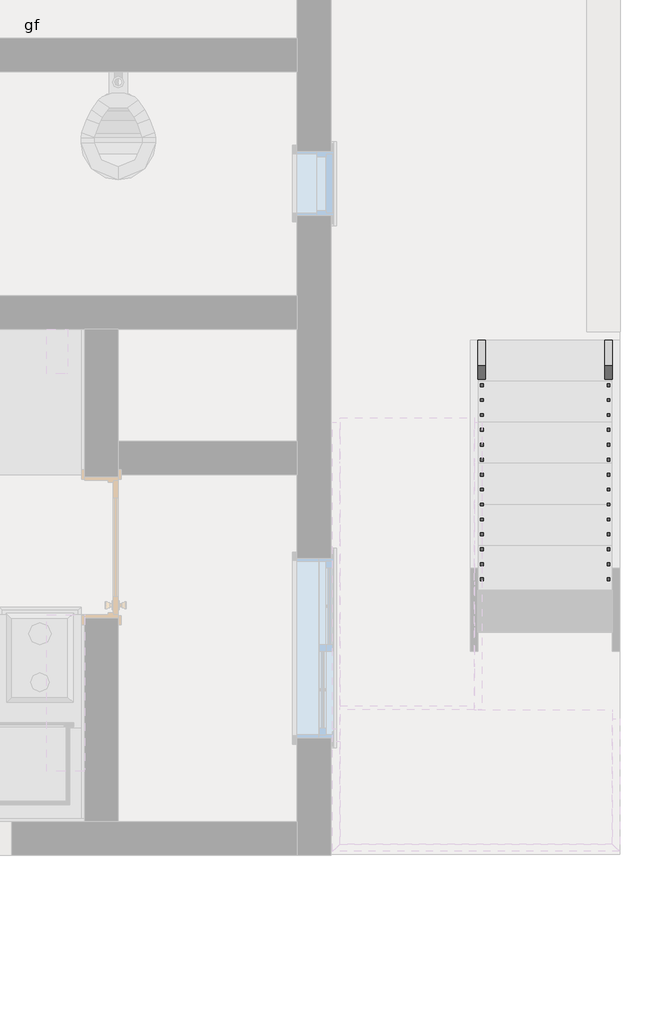
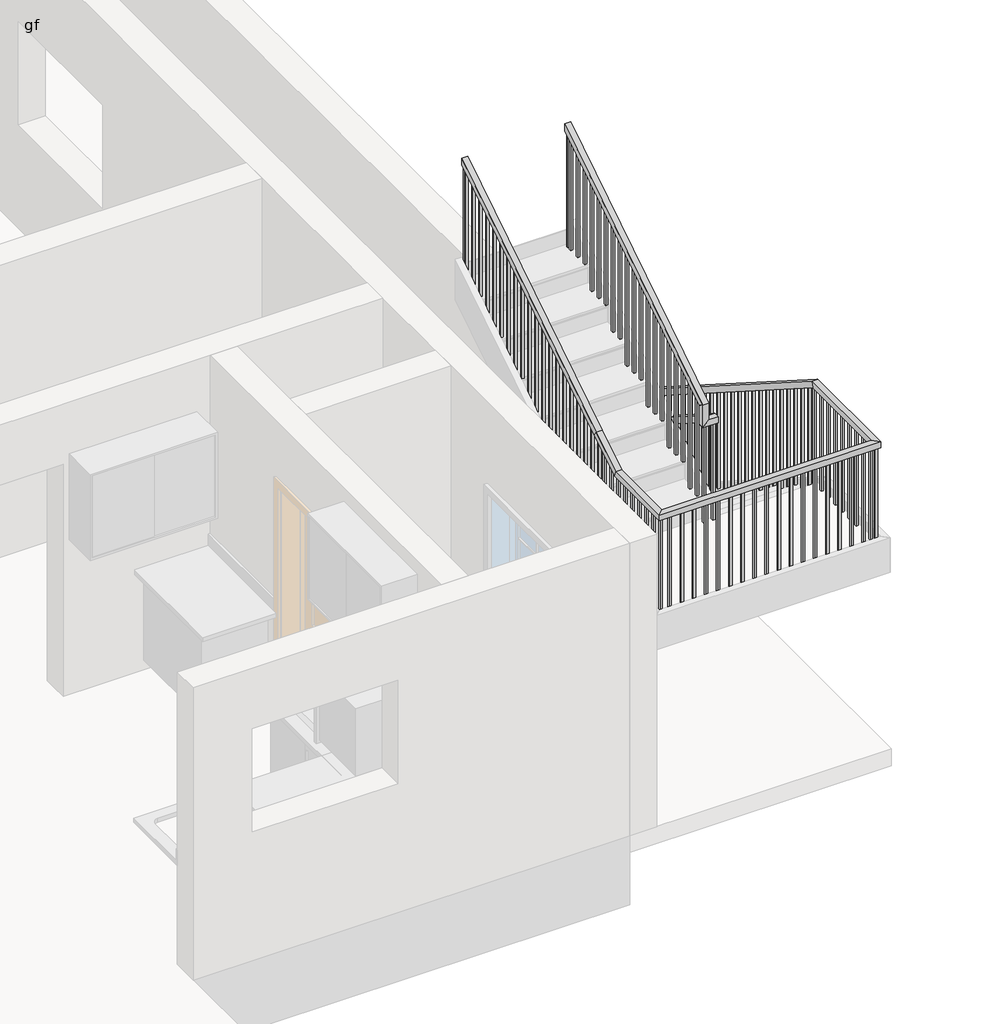
# One storey, part 6 of 8: 2 railings.
"""IFC4 building model written with IfcOpenShell, lengths in millimetres."""

from ifc_helpers import new_model, si_unit, frame, origin, place, context, project, spatial, polyline, outline, extrude, faceted_brep, element, save

model = new_model("IFC4")

# Units and contexts
model_context = context("Model", 3, world=origin())
ifc_project = project(units=[si_unit("LENGTHUNIT", "METRE", prefix="MILLI")], contexts=[model_context])

# Site, building, storey
site = spatial("IfcSite", under=ifc_project)
building = spatial("IfcBuilding", under=site)
storey = spatial("IfcBuildingStorey", under=building, Name="gf", Elevation=609.6)

# Railings
placement = place(None, origin())
element("IfcRailing", 1, ObjectType="Handrail - Rectangular", at=placement, inside=storey, context=model_context, shape_type="SolidModel", body=[
    faceted_brep([(14286.6761273, -1100.1064015, 1701.8), (14286.6761273, -1100.1064015, 1641.586276), (14235.8761273, -1100.1064015, 1641.586276), (14235.8761273, -1100.1064015, 1701.8), (14286.6761273, -3614.7064015, 3302.0), (14235.8761273, -3614.7064015, 3302.0), (14235.8761273, -3614.7064015, 3241.786276), (14286.6761273, -3614.7064015, 3241.786276)], [[[0, 1, 2, 3]], [[4, 5, 6, 7]], [[1, 0, 4, 7]], [[2, 1, 7, 6]], [[3, 2, 6, 5]], [[0, 3, 5, 4]]]),
    faceted_brep([(14286.6761273, -3665.5064015, 3302.0), (14286.6761273, -3665.5064015, 3251.2), (14286.6761273, -3614.7064015, 3251.2), (14286.6761273, -3614.7064015, 3302.0), (14210.4761273, -3665.5064015, 3302.0), (14210.4761273, -3614.7064015, 3302.0), (14159.6761273, -3614.7064015, 3251.2), (14159.6761273, -3665.5064015, 3251.2)], [[[0, 1, 2, 3]], [[4, 5, 6, 7]], [[1, 0, 4, 7]], [[2, 1, 7, 6]], [[3, 2, 6, 5]], [[0, 3, 5, 4]]]),
    faceted_brep([(14210.4761273, -3665.5064015, 3302.0), (14159.6761273, -3665.5064015, 3251.2), (14159.6761273, -3614.7064015, 3251.2), (14210.4761273, -3614.7064015, 3302.0), (14210.4761273, -3665.5064015, 3447.4727273), (14210.4761273, -3614.7064015, 3419.586276), (14159.6761273, -3614.7064015, 3419.586276), (14159.6761273, -3665.5064015, 3447.4727273)], [[[0, 1, 2, 3]], [[4, 5, 6, 7]], [[1, 0, 4, 7]], [[2, 1, 7, 6]], [[3, 2, 6, 5]], [[0, 3, 5, 4]]]),
    faceted_brep([(14159.6761273, -3665.5064015, 3447.4727273), (14159.6761273, -3614.7064015, 3419.586276), (14210.4761273, -3614.7064015, 3419.586276), (14210.4761273, -3665.5064015, 3447.4727273), (14159.6761273, -1658.9064015, 4724.4), (14210.4761273, -1658.9064015, 4724.4), (14210.4761273, -1658.9064015, 4664.186276), (14159.6761273, -1658.9064015, 4664.186276)], [[[0, 1, 2, 3]], [[4, 5, 6, 7]], [[1, 0, 4, 7]], [[2, 1, 7, 6]], [[3, 2, 6, 5]], [[0, 3, 5, 4]]]),
    extrude(outline(polyline([(-1719.2314015, 4625.7976396), (-1700.1814015, 4637.9203669), (-1700.1814015, 3632.2), (-1719.2314015, 3632.2), (-1719.2314015, 4625.7976396)])), frame((14175.5511273, 0.0, 0.0), z_axis=(1.0, 0.0, 0.0), x_axis=(0.0, 1.0, 0.0)), (0.0, 0.0, 1.0), 19.05),
    extrude(outline(polyline([(-1820.8314015, 4561.1430941), (-1801.7814015, 4573.2658214), (-1801.7814015, 3632.2), (-1820.8314015, 3632.2), (-1820.8314015, 4561.1430941)])), frame((14175.5511273, 0.0, 0.0), z_axis=(1.0, 0.0, 0.0), x_axis=(0.0, 1.0, 0.0)), (0.0, 0.0, 1.0), 19.05),
    extrude(outline(polyline([(-1922.4314015, 4496.4885487), (-1903.3814015, 4508.611276), (-1903.3814015, 3632.2), (-1922.4314015, 3632.2), (-1922.4314015, 4496.4885487)])), frame((14175.5511273, 0.0, 0.0), z_axis=(1.0, 0.0, 0.0), x_axis=(0.0, 1.0, 0.0)), (0.0, 0.0, 1.0), 19.05),
    extrude(outline(polyline([(-2024.0314015, 4431.8340032), (-2004.9814015, 4443.9567305), (-2004.9814015, 3454.4), (-2024.0314015, 3454.4), (-2024.0314015, 4431.8340032)])), frame((14175.5511273, 0.0, 0.0), z_axis=(1.0, 0.0, 0.0), x_axis=(0.0, 1.0, 0.0)), (0.0, 0.0, 1.0), 19.05),
    extrude(outline(polyline([(-2125.6314015, 4367.1794578), (-2106.5814015, 4379.3021851), (-2106.5814015, 3454.4), (-2125.6314015, 3454.4), (-2125.6314015, 4367.1794578)])), frame((14175.5511273, 0.0, 0.0), z_axis=(1.0, 0.0, 0.0), x_axis=(0.0, 1.0, 0.0)), (0.0, 0.0, 1.0), 19.05),
    extrude(outline(polyline([(-2227.2314015, 4302.5249123), (-2208.1814015, 4314.6476396), (-2208.1814015, 3454.4), (-2227.2314015, 3454.4), (-2227.2314015, 4302.5249123)])), frame((14175.5511273, 0.0, 0.0), z_axis=(1.0, 0.0, 0.0), x_axis=(0.0, 1.0, 0.0)), (0.0, 0.0, 1.0), 19.05),
    extrude(outline(polyline([(-2328.8314015, 4237.8703669), (-2309.7814015, 4249.9930941), (-2309.7814015, 3276.6), (-2328.8314015, 3276.6), (-2328.8314015, 4237.8703669)])), frame((14175.5511273, 0.0, 0.0), z_axis=(1.0, 0.0, 0.0), x_axis=(0.0, 1.0, 0.0)), (0.0, 0.0, 1.0), 19.05),
    extrude(outline(polyline([(-2430.4314015, 4173.2158214), (-2411.3814015, 4185.3385487), (-2411.3814015, 3276.6), (-2430.4314015, 3276.6), (-2430.4314015, 4173.2158214)])), frame((14175.5511273, 0.0, 0.0), z_axis=(1.0, 0.0, 0.0), x_axis=(0.0, 1.0, 0.0)), (0.0, 0.0, 1.0), 19.05),
    extrude(outline(polyline([(-2532.0314015, 4108.561276), (-2512.9814015, 4120.6840032), (-2512.9814015, 3098.8), (-2532.0314015, 3098.8), (-2532.0314015, 4108.561276)])), frame((14175.5511273, 0.0, 0.0), z_axis=(1.0, 0.0, 0.0), x_axis=(0.0, 1.0, 0.0)), (0.0, 0.0, 1.0), 19.05),
    extrude(outline(polyline([(-2633.6314015, 4043.9067305), (-2614.5814015, 4056.0294578), (-2614.5814015, 3098.8), (-2633.6314015, 3098.8), (-2633.6314015, 4043.9067305)])), frame((14175.5511273, 0.0, 0.0), z_axis=(1.0, 0.0, 0.0), x_axis=(0.0, 1.0, 0.0)), (0.0, 0.0, 1.0), 19.05),
    extrude(outline(polyline([(-2735.2314015, 3979.2521851), (-2716.1814015, 3991.3749123), (-2716.1814015, 3098.8), (-2735.2314015, 3098.8), (-2735.2314015, 3979.2521851)])), frame((14175.5511273, 0.0, 0.0), z_axis=(1.0, 0.0, 0.0), x_axis=(0.0, 1.0, 0.0)), (0.0, 0.0, 1.0), 19.05),
    extrude(outline(polyline([(-2836.8314015, 3914.5976396), (-2817.7814015, 3926.7203669), (-2817.7814015, 2921.0), (-2836.8314015, 2921.0), (-2836.8314015, 3914.5976396)])), frame((14175.5511273, 0.0, 0.0), z_axis=(1.0, 0.0, 0.0), x_axis=(0.0, 1.0, 0.0)), (0.0, 0.0, 1.0), 19.05),
    extrude(outline(polyline([(-2938.4314015, 3849.9430941), (-2919.3814015, 3862.0658214), (-2919.3814015, 2921.0), (-2938.4314015, 2921.0), (-2938.4314015, 3849.9430941)])), frame((14175.5511273, 0.0, 0.0), z_axis=(1.0, 0.0, 0.0), x_axis=(0.0, 1.0, 0.0)), (0.0, 0.0, 1.0), 19.05),
    extrude(outline(polyline([(-3040.0314015, 3785.2885487), (-3020.9814015, 3797.411276), (-3020.9814015, 2921.0), (-3040.0314015, 2921.0), (-3040.0314015, 3785.2885487)])), frame((14175.5511273, 0.0, 0.0), z_axis=(1.0, 0.0, 0.0), x_axis=(0.0, 1.0, 0.0)), (0.0, 0.0, 1.0), 19.05),
    extrude(outline(polyline([(-3141.6314015, 3720.6340032), (-3122.5814015, 3732.7567305), (-3122.5814015, 2743.2), (-3141.6314015, 2743.2), (-3141.6314015, 3720.6340032)])), frame((14175.5511273, 0.0, 0.0), z_axis=(1.0, 0.0, 0.0), x_axis=(0.0, 1.0, 0.0)), (0.0, 0.0, 1.0), 19.05),
    extrude(outline(polyline([(-3243.2314015, 3655.9794578), (-3224.1814015, 3668.1021851), (-3224.1814015, 2743.2), (-3243.2314015, 2743.2), (-3243.2314015, 3655.9794578)])), frame((14175.5511273, 0.0, 0.0), z_axis=(1.0, 0.0, 0.0), x_axis=(0.0, 1.0, 0.0)), (0.0, 0.0, 1.0), 19.05),
    extrude(outline(polyline([(-3344.8314015, 3591.3249123), (-3325.7814015, 3603.4476396), (-3325.7814015, 2743.2), (-3344.8314015, 2743.2), (-3344.8314015, 3591.3249123)])), frame((14175.5511273, 0.0, 0.0), z_axis=(1.0, 0.0, 0.0), x_axis=(0.0, 1.0, 0.0)), (0.0, 0.0, 1.0), 19.05),
    extrude(outline(polyline([(-3446.4314015, 3526.6703669), (-3427.3814015, 3538.7930941), (-3427.3814015, 2565.4), (-3446.4314015, 2565.4), (-3446.4314015, 3526.6703669)])), frame((14175.5511273, 0.0, 0.0), z_axis=(1.0, 0.0, 0.0), x_axis=(0.0, 1.0, 0.0)), (0.0, 0.0, 1.0), 19.05),
    extrude(outline(polyline([(-3548.0314015, 3462.0158214), (-3528.9814015, 3474.1385487), (-3528.9814015, 2565.4), (-3548.0314015, 2565.4), (-3548.0314015, 3462.0158214)])), frame((14175.5511273, 0.0, 0.0), z_axis=(1.0, 0.0, 0.0), x_axis=(0.0, 1.0, 0.0)), (0.0, 0.0, 1.0), 19.05),
    extrude(outline(polyline([(-3548.0314015, 3199.3567305), (-3528.9814015, 3187.2340032), (-3528.9814015, 2209.8), (-3548.0314015, 2209.8), (-3548.0314015, 3199.3567305)])), frame((14251.7511273, 0.0, 0.0), z_axis=(1.0, 0.0, 0.0), x_axis=(0.0, 1.0, 0.0)), (0.0, 0.0, 1.0), 19.05),
    extrude(outline(polyline([(-3446.4314015, 3134.7021851), (-3427.3814015, 3122.5794578), (-3427.3814015, 2209.8), (-3446.4314015, 2209.8), (-3446.4314015, 3134.7021851)])), frame((14251.7511273, 0.0, 0.0), z_axis=(1.0, 0.0, 0.0), x_axis=(0.0, 1.0, 0.0)), (0.0, 0.0, 1.0), 19.05),
    extrude(outline(polyline([(-3344.8314015, 3070.0476396), (-3325.7814015, 3057.9249123), (-3325.7814015, 2209.8), (-3344.8314015, 2209.8), (-3344.8314015, 3070.0476396)])), frame((14251.7511273, 0.0, 0.0), z_axis=(1.0, 0.0, 0.0), x_axis=(0.0, 1.0, 0.0)), (0.0, 0.0, 1.0), 19.05),
    extrude(outline(polyline([(-3243.2314015, 3005.3930941), (-3224.1814015, 2993.2703669), (-3224.1814015, 2032.0), (-3243.2314015, 2032.0), (-3243.2314015, 3005.3930941)])), frame((14251.7511273, 0.0, 0.0), z_axis=(1.0, 0.0, 0.0), x_axis=(0.0, 1.0, 0.0)), (0.0, 0.0, 1.0), 19.05),
    extrude(outline(polyline([(-3141.6314015, 2940.7385487), (-3122.5814015, 2928.6158214), (-3122.5814015, 2032.0), (-3141.6314015, 2032.0), (-3141.6314015, 2940.7385487)])), frame((14251.7511273, 0.0, 0.0), z_axis=(1.0, 0.0, 0.0), x_axis=(0.0, 1.0, 0.0)), (0.0, 0.0, 1.0), 19.05),
    extrude(outline(polyline([(-3040.0314015, 2876.0840032), (-3020.9814015, 2863.961276), (-3020.9814015, 1854.2), (-3040.0314015, 1854.2), (-3040.0314015, 2876.0840032)])), frame((14251.7511273, 0.0, 0.0), z_axis=(1.0, 0.0, 0.0), x_axis=(0.0, 1.0, 0.0)), (0.0, 0.0, 1.0), 19.05),
    extrude(outline(polyline([(-2938.4314015, 2811.4294578), (-2919.3814015, 2799.3067305), (-2919.3814015, 1854.2), (-2938.4314015, 1854.2), (-2938.4314015, 2811.4294578)])), frame((14251.7511273, 0.0, 0.0), z_axis=(1.0, 0.0, 0.0), x_axis=(0.0, 1.0, 0.0)), (0.0, 0.0, 1.0), 19.05),
    extrude(outline(polyline([(-2836.8314015, 2746.7749123), (-2817.7814015, 2734.6521851), (-2817.7814015, 1854.2), (-2836.8314015, 1854.2), (-2836.8314015, 2746.7749123)])), frame((14251.7511273, 0.0, 0.0), z_axis=(1.0, 0.0, 0.0), x_axis=(0.0, 1.0, 0.0)), (0.0, 0.0, 1.0), 19.05),
    extrude(outline(polyline([(-2735.2314015, 2682.1203669), (-2716.1814015, 2669.9976396), (-2716.1814015, 1676.4), (-2735.2314015, 1676.4), (-2735.2314015, 2682.1203669)])), frame((14251.7511273, 0.0, 0.0), z_axis=(1.0, 0.0, 0.0), x_axis=(0.0, 1.0, 0.0)), (0.0, 0.0, 1.0), 19.05),
    extrude(outline(polyline([(-2633.6314015, 2617.4658214), (-2614.5814015, 2605.3430941), (-2614.5814015, 1676.4), (-2633.6314015, 1676.4), (-2633.6314015, 2617.4658214)])), frame((14251.7511273, 0.0, 0.0), z_axis=(1.0, 0.0, 0.0), x_axis=(0.0, 1.0, 0.0)), (0.0, 0.0, 1.0), 19.05),
    extrude(outline(polyline([(-2532.0314015, 2552.811276), (-2512.9814015, 2540.6885487), (-2512.9814015, 1676.4), (-2532.0314015, 1676.4), (-2532.0314015, 2552.811276)])), frame((14251.7511273, 0.0, 0.0), z_axis=(1.0, 0.0, 0.0), x_axis=(0.0, 1.0, 0.0)), (0.0, 0.0, 1.0), 19.05),
    extrude(outline(polyline([(-2430.4314015, 2488.1567305), (-2411.3814015, 2476.0340032), (-2411.3814015, 1498.6), (-2430.4314015, 1498.6), (-2430.4314015, 2488.1567305)])), frame((14251.7511273, 0.0, 0.0), z_axis=(1.0, 0.0, 0.0), x_axis=(0.0, 1.0, 0.0)), (0.0, 0.0, 1.0), 19.05),
    extrude(outline(polyline([(-2328.8314015, 2423.5021851), (-2309.7814015, 2411.3794578), (-2309.7814015, 1498.6), (-2328.8314015, 1498.6), (-2328.8314015, 2423.5021851)])), frame((14251.7511273, 0.0, 0.0), z_axis=(1.0, 0.0, 0.0), x_axis=(0.0, 1.0, 0.0)), (0.0, 0.0, 1.0), 19.05),
    extrude(outline(polyline([(-2227.2314015, 2358.8476396), (-2208.1814015, 2346.7249123), (-2208.1814015, 1498.6), (-2227.2314015, 1498.6), (-2227.2314015, 2358.8476396)])), frame((14251.7511273, 0.0, 0.0), z_axis=(1.0, 0.0, 0.0), x_axis=(0.0, 1.0, 0.0)), (0.0, 0.0, 1.0), 19.05),
    extrude(outline(polyline([(-2125.6314015, 2294.1930941), (-2106.5814015, 2282.0703669), (-2106.5814015, 1320.8), (-2125.6314015, 1320.8), (-2125.6314015, 2294.1930941)])), frame((14251.7511273, 0.0, 0.0), z_axis=(1.0, 0.0, 0.0), x_axis=(0.0, 1.0, 0.0)), (0.0, 0.0, 1.0), 19.05),
    extrude(outline(polyline([(-2024.0314015, 2229.5385487), (-2004.9814015, 2217.4158214), (-2004.9814015, 1320.8), (-2024.0314015, 1320.8), (-2024.0314015, 2229.5385487)])), frame((14251.7511273, 0.0, 0.0), z_axis=(1.0, 0.0, 0.0), x_axis=(0.0, 1.0, 0.0)), (0.0, 0.0, 1.0), 19.05),
    extrude(outline(polyline([(-1922.4314015, 2164.8840032), (-1903.3814015, 2152.761276), (-1903.3814015, 1143.0), (-1922.4314015, 1143.0), (-1922.4314015, 2164.8840032)])), frame((14251.7511273, 0.0, 0.0), z_axis=(1.0, 0.0, 0.0), x_axis=(0.0, 1.0, 0.0)), (0.0, 0.0, 1.0), 19.05),
    extrude(outline(polyline([(-1820.8314015, 2100.2294578), (-1801.7814015, 2088.1067305), (-1801.7814015, 1143.0), (-1820.8314015, 1143.0), (-1820.8314015, 2100.2294578)])), frame((14251.7511273, 0.0, 0.0), z_axis=(1.0, 0.0, 0.0), x_axis=(0.0, 1.0, 0.0)), (0.0, 0.0, 1.0), 19.05),
    extrude(outline(polyline([(-1719.2314015, 2035.5749123), (-1700.1814015, 2023.4521851), (-1700.1814015, 1143.0), (-1719.2314015, 1143.0), (-1719.2314015, 2035.5749123)])), frame((14251.7511273, 0.0, 0.0), z_axis=(1.0, 0.0, 0.0), x_axis=(0.0, 1.0, 0.0)), (0.0, 0.0, 1.0), 19.05),
    extrude(outline(polyline([(-1617.6314015, 1970.9203669), (-1598.5814015, 1958.7976396), (-1598.5814015, 965.2), (-1617.6314015, 965.2), (-1617.6314015, 1970.9203669)])), frame((14251.7511273, 0.0, 0.0), z_axis=(1.0, 0.0, 0.0), x_axis=(0.0, 1.0, 0.0)), (0.0, 0.0, 1.0), 19.05),
    extrude(outline(polyline([(-1516.0314015, 1906.2658214), (-1496.9814015, 1894.1430941), (-1496.9814015, 965.2), (-1516.0314015, 965.2), (-1516.0314015, 1906.2658214)])), frame((14251.7511273, 0.0, 0.0), z_axis=(1.0, 0.0, 0.0), x_axis=(0.0, 1.0, 0.0)), (0.0, 0.0, 1.0), 19.05),
    extrude(outline(polyline([(-1414.4314015, 1841.611276), (-1395.3814015, 1829.4885487), (-1395.3814015, 965.2), (-1414.4314015, 965.2), (-1414.4314015, 1841.611276)])), frame((14251.7511273, 0.0, 0.0), z_axis=(1.0, 0.0, 0.0), x_axis=(0.0, 1.0, 0.0)), (0.0, 0.0, 1.0), 19.05),
    extrude(outline(polyline([(-1312.8314015, 1776.9567305), (-1293.7814015, 1764.8340032), (-1293.7814015, 787.4), (-1312.8314015, 787.4), (-1312.8314015, 1776.9567305)])), frame((14251.7511273, 0.0, 0.0), z_axis=(1.0, 0.0, 0.0), x_axis=(0.0, 1.0, 0.0)), (0.0, 0.0, 1.0), 19.05),
    extrude(outline(polyline([(-1211.2314015, 1712.3021851), (-1192.1814015, 1700.1794578), (-1192.1814015, 787.4), (-1211.2314015, 787.4), (-1211.2314015, 1712.3021851)])), frame((14251.7511273, 0.0, 0.0), z_axis=(1.0, 0.0, 0.0), x_axis=(0.0, 1.0, 0.0)), (0.0, 0.0, 1.0), 19.05),
    extrude(outline(polyline([(14194.6011273, -3630.5814015), (14194.6011273, -3649.6314015), (14175.5511273, -3649.6314015), (14175.5511273, -3630.5814015), (14194.6011273, -3630.5814015)])), frame((0.0, 0.0, 2387.6), z_axis=(0.0, 0.0, 1.0), x_axis=(1.0, 0.0, 0.0)), (0.0, 0.0, 1.0), 863.6),
    extrude(outline(polyline([(-3649.6314015, 3264.011276), (-3630.5814015, 3251.8885487), (-3630.5814015, 2387.6), (-3649.6314015, 2387.6), (-3649.6314015, 3264.011276)])), frame((14251.7511273, 0.0, 0.0), z_axis=(1.0, 0.0, 0.0), x_axis=(0.0, 1.0, 0.0)), (0.0, 0.0, 1.0), 19.05),
    extrude(outline(polyline([(-1677.9564015, 4652.0635487), (-1658.9064015, 4664.186276), (-1658.9064015, 3632.2), (-1677.9564015, 3632.2), (-1677.9564015, 4652.0635487)])), frame((14175.5511273, 0.0, 0.0), z_axis=(1.0, 0.0, 0.0), x_axis=(0.0, 1.0, 0.0)), (0.0, 0.0, 1.0), 19.05),
    extrude(outline(polyline([(-1119.1564015, 1653.7090032), (-1100.1064015, 1641.586276), (-1100.1064015, 787.4), (-1119.1564015, 787.4), (-1119.1564015, 1653.7090032)])), frame((14251.7511273, 0.0, 0.0), z_axis=(1.0, 0.0, 0.0), x_axis=(0.0, 1.0, 0.0)), (0.0, 0.0, 1.0), 19.05),
])
element("IfcRailing", 2, ObjectType="Handrail - Rectangular", at=placement, inside=storey, context=model_context, shape_type="SolidModel", body=[
    faceted_brep([(15150.2761273, -1100.1064015, 1701.8), (15150.2761273, -1100.1064015, 1641.586276), (15099.4761273, -1100.1064015, 1641.586276), (15099.4761273, -1100.1064015, 1701.8), (15150.2761273, -3614.7064015, 3302.0), (15150.2761273, -3629.4993964, 3251.2), (15099.4761273, -3629.4993964, 3251.2), (15099.4761273, -3614.7064015, 3302.0), (15150.2761273, -4529.1064015, 3302.0), (15150.2761273, -4529.1064015, 3251.2), (15099.4761273, -4478.3064015, 3251.2), (15099.4761273, -4478.3064015, 3302.0), (13296.0761273, -4529.1064015, 3302.0), (13296.0761273, -4529.1064015, 3251.2), (13346.8761273, -4478.3064015, 3251.2), (13346.8761273, -4478.3064015, 3302.0), (13296.0761273, -3894.1064015, 3302.0), (13296.0761273, -3879.3134066, 3251.2), (13346.8761273, -3879.3134066, 3251.2), (13346.8761273, -3894.1064015, 3302.0), (13296.0761273, -3614.7064015, 3479.8), (13296.0761273, -3587.4331265, 3436.9419964), (13346.8761273, -3587.4331265, 3436.9419964), (13346.8761273, -3614.7064015, 3479.8), (13296.0761273, -1658.9064015, 4724.4), (13346.8761273, -1658.9064015, 4724.4), (13346.8761273, -1658.9064015, 4664.186276), (13296.0761273, -1658.9064015, 4664.186276)], [[[0, 1, 2, 3]], [[1, 0, 4, 5]], [[2, 1, 5, 6]], [[3, 2, 6, 7]], [[0, 3, 7, 4]], [[5, 4, 8, 9]], [[6, 5, 9, 10]], [[7, 6, 10, 11]], [[4, 7, 11, 8]], [[9, 8, 12, 13]], [[10, 9, 13, 14]], [[11, 10, 14, 15]], [[8, 11, 15, 12]], [[13, 12, 16, 17]], [[14, 13, 17, 18]], [[15, 14, 18, 19]], [[12, 15, 19, 16]], [[17, 16, 20, 21]], [[18, 17, 21, 22]], [[19, 18, 22, 23]], [[16, 19, 23, 20]], [[24, 25, 26, 27]], [[21, 20, 24, 27]], [[22, 21, 27, 26]], [[23, 22, 26, 25]], [[20, 23, 25, 24]]]),
    extrude(outline(polyline([(-1674.7814015, 4654.0840032), (-1674.7814015, 3632.2), (-1693.8314015, 3632.2), (-1693.8314015, 4641.961276), (-1674.7814015, 4654.0840032)])), frame((13311.9511273, 0.0, 0.0), z_axis=(1.0, 0.0, 0.0), x_axis=(0.0, 1.0, 0.0)), (0.0, 0.0, 1.0), 19.05),
    extrude(outline(polyline([(-1776.3814015, 4589.4294578), (-1776.3814015, 3632.2), (-1795.4314015, 3632.2), (-1795.4314015, 4577.3067305), (-1776.3814015, 4589.4294578)])), frame((13311.9511273, 0.0, 0.0), z_axis=(1.0, 0.0, 0.0), x_axis=(0.0, 1.0, 0.0)), (0.0, 0.0, 1.0), 19.05),
    extrude(outline(polyline([(-1877.9814015, 4524.7749123), (-1877.9814015, 3632.2), (-1897.0314015, 3632.2), (-1897.0314015, 4512.6521851), (-1877.9814015, 4524.7749123)])), frame((13311.9511273, 0.0, 0.0), z_axis=(1.0, 0.0, 0.0), x_axis=(0.0, 1.0, 0.0)), (0.0, 0.0, 1.0), 19.05),
    extrude(outline(polyline([(-1979.5814015, 4460.1203669), (-1979.5814015, 3454.4), (-1998.6314015, 3454.4), (-1998.6314015, 4447.9976396), (-1979.5814015, 4460.1203669)])), frame((13311.9511273, 0.0, 0.0), z_axis=(1.0, 0.0, 0.0), x_axis=(0.0, 1.0, 0.0)), (0.0, 0.0, 1.0), 19.05),
    extrude(outline(polyline([(-2081.1814015, 4395.4658214), (-2081.1814015, 3454.4), (-2100.2314015, 3454.4), (-2100.2314015, 4383.3430941), (-2081.1814015, 4395.4658214)])), frame((13311.9511273, 0.0, 0.0), z_axis=(1.0, 0.0, 0.0), x_axis=(0.0, 1.0, 0.0)), (0.0, 0.0, 1.0), 19.05),
    extrude(outline(polyline([(-2182.7814015, 4330.811276), (-2182.7814015, 3454.4), (-2201.8314015, 3454.4), (-2201.8314015, 4318.6885487), (-2182.7814015, 4330.811276)])), frame((13311.9511273, 0.0, 0.0), z_axis=(1.0, 0.0, 0.0), x_axis=(0.0, 1.0, 0.0)), (0.0, 0.0, 1.0), 19.05),
    extrude(outline(polyline([(-2284.3814015, 4266.1567305), (-2284.3814015, 3276.6), (-2303.4314015, 3276.6), (-2303.4314015, 4254.0340032), (-2284.3814015, 4266.1567305)])), frame((13311.9511273, 0.0, 0.0), z_axis=(1.0, 0.0, 0.0), x_axis=(0.0, 1.0, 0.0)), (0.0, 0.0, 1.0), 19.05),
    extrude(outline(polyline([(-2385.9814015, 4201.5021851), (-2385.9814015, 3276.6), (-2405.0314015, 3276.6), (-2405.0314015, 4189.3794578), (-2385.9814015, 4201.5021851)])), frame((13311.9511273, 0.0, 0.0), z_axis=(1.0, 0.0, 0.0), x_axis=(0.0, 1.0, 0.0)), (0.0, 0.0, 1.0), 19.05),
    extrude(outline(polyline([(-2487.5814015, 4136.8476396), (-2487.5814015, 3276.6), (-2506.6314015, 3276.6), (-2506.6314015, 4124.7249123), (-2487.5814015, 4136.8476396)])), frame((13311.9511273, 0.0, 0.0), z_axis=(1.0, 0.0, 0.0), x_axis=(0.0, 1.0, 0.0)), (0.0, 0.0, 1.0), 19.05),
    extrude(outline(polyline([(-2589.1814015, 4072.1930941), (-2589.1814015, 3098.8), (-2608.2314015, 3098.8), (-2608.2314015, 4060.0703669), (-2589.1814015, 4072.1930941)])), frame((13311.9511273, 0.0, 0.0), z_axis=(1.0, 0.0, 0.0), x_axis=(0.0, 1.0, 0.0)), (0.0, 0.0, 1.0), 19.05),
    extrude(outline(polyline([(-2690.7814015, 4007.5385487), (-2690.7814015, 3098.8), (-2709.8314015, 3098.8), (-2709.8314015, 3995.4158214), (-2690.7814015, 4007.5385487)])), frame((13311.9511273, 0.0, 0.0), z_axis=(1.0, 0.0, 0.0), x_axis=(0.0, 1.0, 0.0)), (0.0, 0.0, 1.0), 19.05),
    extrude(outline(polyline([(-2792.3814015, 3942.8840032), (-2792.3814015, 2921.0), (-2811.4314015, 2921.0), (-2811.4314015, 3930.761276), (-2792.3814015, 3942.8840032)])), frame((13311.9511273, 0.0, 0.0), z_axis=(1.0, 0.0, 0.0), x_axis=(0.0, 1.0, 0.0)), (0.0, 0.0, 1.0), 19.05),
    extrude(outline(polyline([(-2893.9814015, 3878.2294578), (-2893.9814015, 2921.0), (-2913.0314015, 2921.0), (-2913.0314015, 3866.1067305), (-2893.9814015, 3878.2294578)])), frame((13311.9511273, 0.0, 0.0), z_axis=(1.0, 0.0, 0.0), x_axis=(0.0, 1.0, 0.0)), (0.0, 0.0, 1.0), 19.05),
    extrude(outline(polyline([(-2995.5814015, 3813.5749123), (-2995.5814015, 2921.0), (-3014.6314015, 2921.0), (-3014.6314015, 3801.4521851), (-2995.5814015, 3813.5749123)])), frame((13311.9511273, 0.0, 0.0), z_axis=(1.0, 0.0, 0.0), x_axis=(0.0, 1.0, 0.0)), (0.0, 0.0, 1.0), 19.05),
    extrude(outline(polyline([(-3097.1814015, 3748.9203669), (-3097.1814015, 2743.2), (-3116.2314015, 2743.2), (-3116.2314015, 3736.7976396), (-3097.1814015, 3748.9203669)])), frame((13311.9511273, 0.0, 0.0), z_axis=(1.0, 0.0, 0.0), x_axis=(0.0, 1.0, 0.0)), (0.0, 0.0, 1.0), 19.05),
    extrude(outline(polyline([(-3198.7814015, 3684.2658214), (-3198.7814015, 2743.2), (-3217.8314015, 2743.2), (-3217.8314015, 3672.1430941), (-3198.7814015, 3684.2658214)])), frame((13311.9511273, 0.0, 0.0), z_axis=(1.0, 0.0, 0.0), x_axis=(0.0, 1.0, 0.0)), (0.0, 0.0, 1.0), 19.05),
    extrude(outline(polyline([(-3300.3814015, 3619.611276), (-3300.3814015, 2743.2), (-3319.4314015, 2743.2), (-3319.4314015, 3607.4885487), (-3300.3814015, 3619.611276)])), frame((13311.9511273, 0.0, 0.0), z_axis=(1.0, 0.0, 0.0), x_axis=(0.0, 1.0, 0.0)), (0.0, 0.0, 1.0), 19.05),
    extrude(outline(polyline([(-3401.9814015, 3554.9567305), (-3401.9814015, 2565.4), (-3421.0314015, 2565.4), (-3421.0314015, 3542.8340032), (-3401.9814015, 3554.9567305)])), frame((13311.9511273, 0.0, 0.0), z_axis=(1.0, 0.0, 0.0), x_axis=(0.0, 1.0, 0.0)), (0.0, 0.0, 1.0), 19.05),
    extrude(outline(polyline([(-3503.5814015, 3490.3021851), (-3503.5814015, 2565.4), (-3522.6314015, 2565.4), (-3522.6314015, 3478.1794578), (-3503.5814015, 3490.3021851)])), frame((13311.9511273, 0.0, 0.0), z_axis=(1.0, 0.0, 0.0), x_axis=(0.0, 1.0, 0.0)), (0.0, 0.0, 1.0), 19.05),
    extrude(outline(polyline([(-3681.3814015, 3377.1567305), (-3681.3814015, 2387.6), (-3700.4314015, 2387.6), (-3700.4314015, 3365.0340032), (-3681.3814015, 3377.1567305)])), frame((13311.9511273, 0.0, 0.0), z_axis=(1.0, 0.0, 0.0), x_axis=(0.0, 1.0, 0.0)), (0.0, 0.0, 1.0), 19.05),
    extrude(outline(polyline([(-3782.9814015, 3312.5021851), (-3782.9814015, 2387.6), (-3802.0314015, 2387.6), (-3802.0314015, 3300.3794578), (-3782.9814015, 3312.5021851)])), frame((13311.9511273, 0.0, 0.0), z_axis=(1.0, 0.0, 0.0), x_axis=(0.0, 1.0, 0.0)), (0.0, 0.0, 1.0), 19.05),
    extrude(outline(polyline([(13311.9511273, -3903.6314015), (13311.9511273, -3884.5814015), (13331.0011273, -3884.5814015), (13331.0011273, -3903.6314015), (13311.9511273, -3903.6314015)])), frame((0.0, 0.0, 2387.6), z_axis=(0.0, 0.0, 1.0), x_axis=(1.0, 0.0, 0.0)), (0.0, 0.0, 1.0), 863.6),
    extrude(outline(polyline([(13311.9511273, -4005.2314015), (13311.9511273, -3986.1814015), (13331.0011273, -3986.1814015), (13331.0011273, -4005.2314015), (13311.9511273, -4005.2314015)])), frame((0.0, 0.0, 2387.6), z_axis=(0.0, 0.0, 1.0), x_axis=(1.0, 0.0, 0.0)), (0.0, 0.0, 1.0), 863.6),
    extrude(outline(polyline([(13311.9511273, -4106.8314015), (13311.9511273, -4087.7814015), (13331.0011273, -4087.7814015), (13331.0011273, -4106.8314015), (13311.9511273, -4106.8314015)])), frame((0.0, 0.0, 2387.6), z_axis=(0.0, 0.0, 1.0), x_axis=(1.0, 0.0, 0.0)), (0.0, 0.0, 1.0), 863.6),
    extrude(outline(polyline([(13311.9511273, -4208.4314015), (13311.9511273, -4189.3814015), (13331.0011273, -4189.3814015), (13331.0011273, -4208.4314015), (13311.9511273, -4208.4314015)])), frame((0.0, 0.0, 2387.6), z_axis=(0.0, 0.0, 1.0), x_axis=(1.0, 0.0, 0.0)), (0.0, 0.0, 1.0), 863.6),
    extrude(outline(polyline([(13311.9511273, -4310.0314015), (13311.9511273, -4290.9814015), (13331.0011273, -4290.9814015), (13331.0011273, -4310.0314015), (13311.9511273, -4310.0314015)])), frame((0.0, 0.0, 2387.6), z_axis=(0.0, 0.0, 1.0), x_axis=(1.0, 0.0, 0.0)), (0.0, 0.0, 1.0), 863.6),
    extrude(outline(polyline([(13311.9511273, -4411.6314015), (13311.9511273, -4392.5814015), (13331.0011273, -4392.5814015), (13331.0011273, -4411.6314015), (13311.9511273, -4411.6314015)])), frame((0.0, 0.0, 2387.6), z_axis=(0.0, 0.0, 1.0), x_axis=(1.0, 0.0, 0.0)), (0.0, 0.0, 1.0), 863.6),
    extrude(outline(polyline([(13407.2011273, -4513.2314015), (13388.1511273, -4513.2314015), (13388.1511273, -4494.1814015), (13407.2011273, -4494.1814015), (13407.2011273, -4513.2314015)])), frame((0.0, 0.0, 2387.6), z_axis=(0.0, 0.0, 1.0), x_axis=(1.0, 0.0, 0.0)), (0.0, 0.0, 1.0), 863.6),
    extrude(outline(polyline([(13508.8011273, -4513.2314015), (13489.7511273, -4513.2314015), (13489.7511273, -4494.1814015), (13508.8011273, -4494.1814015), (13508.8011273, -4513.2314015)])), frame((0.0, 0.0, 2387.6), z_axis=(0.0, 0.0, 1.0), x_axis=(1.0, 0.0, 0.0)), (0.0, 0.0, 1.0), 863.6),
    extrude(outline(polyline([(13610.4011273, -4513.2314015), (13591.3511273, -4513.2314015), (13591.3511273, -4494.1814015), (13610.4011273, -4494.1814015), (13610.4011273, -4513.2314015)])), frame((0.0, 0.0, 2387.6), z_axis=(0.0, 0.0, 1.0), x_axis=(1.0, 0.0, 0.0)), (0.0, 0.0, 1.0), 863.6),
    extrude(outline(polyline([(13712.0011273, -4513.2314015), (13692.9511273, -4513.2314015), (13692.9511273, -4494.1814015), (13712.0011273, -4494.1814015), (13712.0011273, -4513.2314015)])), frame((0.0, 0.0, 2387.6), z_axis=(0.0, 0.0, 1.0), x_axis=(1.0, 0.0, 0.0)), (0.0, 0.0, 1.0), 863.6),
    extrude(outline(polyline([(13813.6011273, -4513.2314015), (13794.5511273, -4513.2314015), (13794.5511273, -4494.1814015), (13813.6011273, -4494.1814015), (13813.6011273, -4513.2314015)])), frame((0.0, 0.0, 2387.6), z_axis=(0.0, 0.0, 1.0), x_axis=(1.0, 0.0, 0.0)), (0.0, 0.0, 1.0), 863.6),
    extrude(outline(polyline([(13915.2011273, -4513.2314015), (13896.1511273, -4513.2314015), (13896.1511273, -4494.1814015), (13915.2011273, -4494.1814015), (13915.2011273, -4513.2314015)])), frame((0.0, 0.0, 2387.6), z_axis=(0.0, 0.0, 1.0), x_axis=(1.0, 0.0, 0.0)), (0.0, 0.0, 1.0), 863.6),
    extrude(outline(polyline([(14016.8011273, -4513.2314015), (13997.7511273, -4513.2314015), (13997.7511273, -4494.1814015), (14016.8011273, -4494.1814015), (14016.8011273, -4513.2314015)])), frame((0.0, 0.0, 2387.6), z_axis=(0.0, 0.0, 1.0), x_axis=(1.0, 0.0, 0.0)), (0.0, 0.0, 1.0), 863.6),
    extrude(outline(polyline([(14118.4011273, -4513.2314015), (14099.3511273, -4513.2314015), (14099.3511273, -4494.1814015), (14118.4011273, -4494.1814015), (14118.4011273, -4513.2314015)])), frame((0.0, 0.0, 2387.6), z_axis=(0.0, 0.0, 1.0), x_axis=(1.0, 0.0, 0.0)), (0.0, 0.0, 1.0), 863.6),
    extrude(outline(polyline([(14220.0011273, -4513.2314015), (14200.9511273, -4513.2314015), (14200.9511273, -4494.1814015), (14220.0011273, -4494.1814015), (14220.0011273, -4513.2314015)])), frame((0.0, 0.0, 2387.6), z_axis=(0.0, 0.0, 1.0), x_axis=(1.0, 0.0, 0.0)), (0.0, 0.0, 1.0), 863.6),
    extrude(outline(polyline([(14321.6011273, -4513.2314015), (14302.5511273, -4513.2314015), (14302.5511273, -4494.1814015), (14321.6011273, -4494.1814015), (14321.6011273, -4513.2314015)])), frame((0.0, 0.0, 2387.6), z_axis=(0.0, 0.0, 1.0), x_axis=(1.0, 0.0, 0.0)), (0.0, 0.0, 1.0), 863.6),
    extrude(outline(polyline([(14423.2011273, -4513.2314015), (14404.1511273, -4513.2314015), (14404.1511273, -4494.1814015), (14423.2011273, -4494.1814015), (14423.2011273, -4513.2314015)])), frame((0.0, 0.0, 2387.6), z_axis=(0.0, 0.0, 1.0), x_axis=(1.0, 0.0, 0.0)), (0.0, 0.0, 1.0), 863.6),
    extrude(outline(polyline([(14524.8011273, -4513.2314015), (14505.7511273, -4513.2314015), (14505.7511273, -4494.1814015), (14524.8011273, -4494.1814015), (14524.8011273, -4513.2314015)])), frame((0.0, 0.0, 2387.6), z_axis=(0.0, 0.0, 1.0), x_axis=(1.0, 0.0, 0.0)), (0.0, 0.0, 1.0), 863.6),
    extrude(outline(polyline([(14626.4011273, -4513.2314015), (14607.3511273, -4513.2314015), (14607.3511273, -4494.1814015), (14626.4011273, -4494.1814015), (14626.4011273, -4513.2314015)])), frame((0.0, 0.0, 2387.6), z_axis=(0.0, 0.0, 1.0), x_axis=(1.0, 0.0, 0.0)), (0.0, 0.0, 1.0), 863.6),
    extrude(outline(polyline([(14728.0011273, -4513.2314015), (14708.9511273, -4513.2314015), (14708.9511273, -4494.1814015), (14728.0011273, -4494.1814015), (14728.0011273, -4513.2314015)])), frame((0.0, 0.0, 2387.6), z_axis=(0.0, 0.0, 1.0), x_axis=(1.0, 0.0, 0.0)), (0.0, 0.0, 1.0), 863.6),
    extrude(outline(polyline([(14829.6011273, -4513.2314015), (14810.5511273, -4513.2314015), (14810.5511273, -4494.1814015), (14829.6011273, -4494.1814015), (14829.6011273, -4513.2314015)])), frame((0.0, 0.0, 2387.6), z_axis=(0.0, 0.0, 1.0), x_axis=(1.0, 0.0, 0.0)), (0.0, 0.0, 1.0), 863.6),
    extrude(outline(polyline([(14931.2011273, -4513.2314015), (14912.1511273, -4513.2314015), (14912.1511273, -4494.1814015), (14931.2011273, -4494.1814015), (14931.2011273, -4513.2314015)])), frame((0.0, 0.0, 2387.6), z_axis=(0.0, 0.0, 1.0), x_axis=(1.0, 0.0, 0.0)), (0.0, 0.0, 1.0), 863.6),
    extrude(outline(polyline([(15032.8011273, -4513.2314015), (15013.7511273, -4513.2314015), (15013.7511273, -4494.1814015), (15032.8011273, -4494.1814015), (15032.8011273, -4513.2314015)])), frame((0.0, 0.0, 2387.6), z_axis=(0.0, 0.0, 1.0), x_axis=(1.0, 0.0, 0.0)), (0.0, 0.0, 1.0), 863.6),
    extrude(outline(polyline([(15134.4011273, -4417.9814015), (15134.4011273, -4437.0314015), (15115.3511273, -4437.0314015), (15115.3511273, -4417.9814015), (15134.4011273, -4417.9814015)])), frame((0.0, 0.0, 2387.6), z_axis=(0.0, 0.0, 1.0), x_axis=(1.0, 0.0, 0.0)), (0.0, 0.0, 1.0), 863.6),
    extrude(outline(polyline([(15134.4011273, -4316.3814015), (15134.4011273, -4335.4314015), (15115.3511273, -4335.4314015), (15115.3511273, -4316.3814015), (15134.4011273, -4316.3814015)])), frame((0.0, 0.0, 2387.6), z_axis=(0.0, 0.0, 1.0), x_axis=(1.0, 0.0, 0.0)), (0.0, 0.0, 1.0), 863.6),
    extrude(outline(polyline([(15134.4011273, -4214.7814015), (15134.4011273, -4233.8314015), (15115.3511273, -4233.8314015), (15115.3511273, -4214.7814015), (15134.4011273, -4214.7814015)])), frame((0.0, 0.0, 2387.6), z_axis=(0.0, 0.0, 1.0), x_axis=(1.0, 0.0, 0.0)), (0.0, 0.0, 1.0), 863.6),
    extrude(outline(polyline([(15134.4011273, -4113.1814015), (15134.4011273, -4132.2314015), (15115.3511273, -4132.2314015), (15115.3511273, -4113.1814015), (15134.4011273, -4113.1814015)])), frame((0.0, 0.0, 2387.6), z_axis=(0.0, 0.0, 1.0), x_axis=(1.0, 0.0, 0.0)), (0.0, 0.0, 1.0), 863.6),
    extrude(outline(polyline([(15134.4011273, -4011.5814015), (15134.4011273, -4030.6314015), (15115.3511273, -4030.6314015), (15115.3511273, -4011.5814015), (15134.4011273, -4011.5814015)])), frame((0.0, 0.0, 2387.6), z_axis=(0.0, 0.0, 1.0), x_axis=(1.0, 0.0, 0.0)), (0.0, 0.0, 1.0), 863.6),
    extrude(outline(polyline([(15134.4011273, -3909.9814015), (15134.4011273, -3929.0314015), (15115.3511273, -3929.0314015), (15115.3511273, -3909.9814015), (15134.4011273, -3909.9814015)])), frame((0.0, 0.0, 2387.6), z_axis=(0.0, 0.0, 1.0), x_axis=(1.0, 0.0, 0.0)), (0.0, 0.0, 1.0), 863.6),
    extrude(outline(polyline([(15134.4011273, -3808.3814015), (15134.4011273, -3827.4314015), (15115.3511273, -3827.4314015), (15115.3511273, -3808.3814015), (15134.4011273, -3808.3814015)])), frame((0.0, 0.0, 2387.6), z_axis=(0.0, 0.0, 1.0), x_axis=(1.0, 0.0, 0.0)), (0.0, 0.0, 1.0), 863.6),
    extrude(outline(polyline([(15134.4011273, -3706.7814015), (15134.4011273, -3725.8314015), (15115.3511273, -3725.8314015), (15115.3511273, -3706.7814015), (15134.4011273, -3706.7814015)])), frame((0.0, 0.0, 2387.6), z_axis=(0.0, 0.0, 1.0), x_axis=(1.0, 0.0, 0.0)), (0.0, 0.0, 1.0), 863.6),
    extrude(outline(polyline([(-3528.9814015, 3187.2340032), (-3528.9814015, 2209.8), (-3548.0314015, 2209.8), (-3548.0314015, 3199.3567305), (-3528.9814015, 3187.2340032)])), frame((15115.3511273, 0.0, 0.0), z_axis=(1.0, 0.0, 0.0), x_axis=(0.0, 1.0, 0.0)), (0.0, 0.0, 1.0), 19.05),
    extrude(outline(polyline([(-3427.3814015, 3122.5794578), (-3427.3814015, 2209.8), (-3446.4314015, 2209.8), (-3446.4314015, 3134.7021851), (-3427.3814015, 3122.5794578)])), frame((15115.3511273, 0.0, 0.0), z_axis=(1.0, 0.0, 0.0), x_axis=(0.0, 1.0, 0.0)), (0.0, 0.0, 1.0), 19.05),
    extrude(outline(polyline([(-3325.7814015, 3057.9249123), (-3325.7814015, 2209.8), (-3344.8314015, 2209.8), (-3344.8314015, 3070.0476396), (-3325.7814015, 3057.9249123)])), frame((15115.3511273, 0.0, 0.0), z_axis=(1.0, 0.0, 0.0), x_axis=(0.0, 1.0, 0.0)), (0.0, 0.0, 1.0), 19.05),
    extrude(outline(polyline([(-3224.1814015, 2993.2703669), (-3224.1814015, 2032.0), (-3243.2314015, 2032.0), (-3243.2314015, 3005.3930941), (-3224.1814015, 2993.2703669)])), frame((15115.3511273, 0.0, 0.0), z_axis=(1.0, 0.0, 0.0), x_axis=(0.0, 1.0, 0.0)), (0.0, 0.0, 1.0), 19.05),
    extrude(outline(polyline([(-3122.5814015, 2928.6158214), (-3122.5814015, 2032.0), (-3141.6314015, 2032.0), (-3141.6314015, 2940.7385487), (-3122.5814015, 2928.6158214)])), frame((15115.3511273, 0.0, 0.0), z_axis=(1.0, 0.0, 0.0), x_axis=(0.0, 1.0, 0.0)), (0.0, 0.0, 1.0), 19.05),
    extrude(outline(polyline([(-3020.9814015, 2863.961276), (-3020.9814015, 1854.2), (-3040.0314015, 1854.2), (-3040.0314015, 2876.0840032), (-3020.9814015, 2863.961276)])), frame((15115.3511273, 0.0, 0.0), z_axis=(1.0, 0.0, 0.0), x_axis=(0.0, 1.0, 0.0)), (0.0, 0.0, 1.0), 19.05),
    extrude(outline(polyline([(-2919.3814015, 2799.3067305), (-2919.3814015, 1854.2), (-2938.4314015, 1854.2), (-2938.4314015, 2811.4294578), (-2919.3814015, 2799.3067305)])), frame((15115.3511273, 0.0, 0.0), z_axis=(1.0, 0.0, 0.0), x_axis=(0.0, 1.0, 0.0)), (0.0, 0.0, 1.0), 19.05),
    extrude(outline(polyline([(-2817.7814015, 2734.6521851), (-2817.7814015, 1854.2), (-2836.8314015, 1854.2), (-2836.8314015, 2746.7749123), (-2817.7814015, 2734.6521851)])), frame((15115.3511273, 0.0, 0.0), z_axis=(1.0, 0.0, 0.0), x_axis=(0.0, 1.0, 0.0)), (0.0, 0.0, 1.0), 19.05),
    extrude(outline(polyline([(-2716.1814015, 2669.9976396), (-2716.1814015, 1676.4), (-2735.2314015, 1676.4), (-2735.2314015, 2682.1203669), (-2716.1814015, 2669.9976396)])), frame((15115.3511273, 0.0, 0.0), z_axis=(1.0, 0.0, 0.0), x_axis=(0.0, 1.0, 0.0)), (0.0, 0.0, 1.0), 19.05),
    extrude(outline(polyline([(-2614.5814015, 2605.3430941), (-2614.5814015, 1676.4), (-2633.6314015, 1676.4), (-2633.6314015, 2617.4658214), (-2614.5814015, 2605.3430941)])), frame((15115.3511273, 0.0, 0.0), z_axis=(1.0, 0.0, 0.0), x_axis=(0.0, 1.0, 0.0)), (0.0, 0.0, 1.0), 19.05),
    extrude(outline(polyline([(-2512.9814015, 2540.6885487), (-2512.9814015, 1676.4), (-2532.0314015, 1676.4), (-2532.0314015, 2552.811276), (-2512.9814015, 2540.6885487)])), frame((15115.3511273, 0.0, 0.0), z_axis=(1.0, 0.0, 0.0), x_axis=(0.0, 1.0, 0.0)), (0.0, 0.0, 1.0), 19.05),
    extrude(outline(polyline([(-2411.3814015, 2476.0340032), (-2411.3814015, 1498.6), (-2430.4314015, 1498.6), (-2430.4314015, 2488.1567305), (-2411.3814015, 2476.0340032)])), frame((15115.3511273, 0.0, 0.0), z_axis=(1.0, 0.0, 0.0), x_axis=(0.0, 1.0, 0.0)), (0.0, 0.0, 1.0), 19.05),
    extrude(outline(polyline([(-2309.7814015, 2411.3794578), (-2309.7814015, 1498.6), (-2328.8314015, 1498.6), (-2328.8314015, 2423.5021851), (-2309.7814015, 2411.3794578)])), frame((15115.3511273, 0.0, 0.0), z_axis=(1.0, 0.0, 0.0), x_axis=(0.0, 1.0, 0.0)), (0.0, 0.0, 1.0), 19.05),
    extrude(outline(polyline([(-2208.1814015, 2346.7249123), (-2208.1814015, 1498.6), (-2227.2314015, 1498.6), (-2227.2314015, 2358.8476396), (-2208.1814015, 2346.7249123)])), frame((15115.3511273, 0.0, 0.0), z_axis=(1.0, 0.0, 0.0), x_axis=(0.0, 1.0, 0.0)), (0.0, 0.0, 1.0), 19.05),
    extrude(outline(polyline([(-2106.5814015, 2282.0703669), (-2106.5814015, 1320.8), (-2125.6314015, 1320.8), (-2125.6314015, 2294.1930941), (-2106.5814015, 2282.0703669)])), frame((15115.3511273, 0.0, 0.0), z_axis=(1.0, 0.0, 0.0), x_axis=(0.0, 1.0, 0.0)), (0.0, 0.0, 1.0), 19.05),
    extrude(outline(polyline([(-2004.9814015, 2217.4158214), (-2004.9814015, 1320.8), (-2024.0314015, 1320.8), (-2024.0314015, 2229.5385487), (-2004.9814015, 2217.4158214)])), frame((15115.3511273, 0.0, 0.0), z_axis=(1.0, 0.0, 0.0), x_axis=(0.0, 1.0, 0.0)), (0.0, 0.0, 1.0), 19.05),
    extrude(outline(polyline([(-1903.3814015, 2152.761276), (-1903.3814015, 1143.0), (-1922.4314015, 1143.0), (-1922.4314015, 2164.8840032), (-1903.3814015, 2152.761276)])), frame((15115.3511273, 0.0, 0.0), z_axis=(1.0, 0.0, 0.0), x_axis=(0.0, 1.0, 0.0)), (0.0, 0.0, 1.0), 19.05),
    extrude(outline(polyline([(-1801.7814015, 2088.1067305), (-1801.7814015, 1143.0), (-1820.8314015, 1143.0), (-1820.8314015, 2100.2294578), (-1801.7814015, 2088.1067305)])), frame((15115.3511273, 0.0, 0.0), z_axis=(1.0, 0.0, 0.0), x_axis=(0.0, 1.0, 0.0)), (0.0, 0.0, 1.0), 19.05),
    extrude(outline(polyline([(-1700.1814015, 2023.4521851), (-1700.1814015, 1143.0), (-1719.2314015, 1143.0), (-1719.2314015, 2035.5749123), (-1700.1814015, 2023.4521851)])), frame((15115.3511273, 0.0, 0.0), z_axis=(1.0, 0.0, 0.0), x_axis=(0.0, 1.0, 0.0)), (0.0, 0.0, 1.0), 19.05),
    extrude(outline(polyline([(-1598.5814015, 1958.7976396), (-1598.5814015, 965.2), (-1617.6314015, 965.2), (-1617.6314015, 1970.9203669), (-1598.5814015, 1958.7976396)])), frame((15115.3511273, 0.0, 0.0), z_axis=(1.0, 0.0, 0.0), x_axis=(0.0, 1.0, 0.0)), (0.0, 0.0, 1.0), 19.05),
    extrude(outline(polyline([(-1496.9814015, 1894.1430941), (-1496.9814015, 965.2), (-1516.0314015, 965.2), (-1516.0314015, 1906.2658214), (-1496.9814015, 1894.1430941)])), frame((15115.3511273, 0.0, 0.0), z_axis=(1.0, 0.0, 0.0), x_axis=(0.0, 1.0, 0.0)), (0.0, 0.0, 1.0), 19.05),
    extrude(outline(polyline([(-1395.3814015, 1829.4885487), (-1395.3814015, 965.2), (-1414.4314015, 965.2), (-1414.4314015, 1841.611276), (-1395.3814015, 1829.4885487)])), frame((15115.3511273, 0.0, 0.0), z_axis=(1.0, 0.0, 0.0), x_axis=(0.0, 1.0, 0.0)), (0.0, 0.0, 1.0), 19.05),
    extrude(outline(polyline([(-1293.7814015, 1764.8340032), (-1293.7814015, 787.4), (-1312.8314015, 787.4), (-1312.8314015, 1776.9567305), (-1293.7814015, 1764.8340032)])), frame((15115.3511273, 0.0, 0.0), z_axis=(1.0, 0.0, 0.0), x_axis=(0.0, 1.0, 0.0)), (0.0, 0.0, 1.0), 19.05),
    extrude(outline(polyline([(-1192.1814015, 1700.1794578), (-1192.1814015, 787.4), (-1211.2314015, 787.4), (-1211.2314015, 1712.3021851), (-1192.1814015, 1700.1794578)])), frame((15115.3511273, 0.0, 0.0), z_axis=(1.0, 0.0, 0.0), x_axis=(0.0, 1.0, 0.0)), (0.0, 0.0, 1.0), 19.05),
    extrude(outline(polyline([(-3605.1814015, 3425.6476396), (-3605.1814015, 2387.6), (-3624.2314015, 2387.6), (-3624.2314015, 3413.5249123), (-3605.1814015, 3425.6476396)])), frame((13311.9511273, 0.0, 0.0), z_axis=(1.0, 0.0, 0.0), x_axis=(0.0, 1.0, 0.0)), (0.0, 0.0, 1.0), 19.05),
    extrude(outline(polyline([(13331.0011273, -4513.2314015), (13311.9511273, -4513.2314015), (13311.9511273, -4494.1814015), (13331.0011273, -4494.1814015), (13331.0011273, -4513.2314015)])), frame((0.0, 0.0, 2387.6), z_axis=(0.0, 0.0, 1.0), x_axis=(1.0, 0.0, 0.0)), (0.0, 0.0, 1.0), 863.6),
    extrude(outline(polyline([(15134.4011273, -4494.1814015), (15134.4011273, -4513.2314015), (15115.3511273, -4513.2314015), (15115.3511273, -4494.1814015), (15134.4011273, -4494.1814015)])), frame((0.0, 0.0, 2387.6), z_axis=(0.0, 0.0, 1.0), x_axis=(1.0, 0.0, 0.0)), (0.0, 0.0, 1.0), 863.6),
    extrude(outline(polyline([(-3605.1814015, 3235.7249123), (-3605.1814015, 2387.6), (-3624.2314015, 2387.6), (-3624.2314015, 3247.8476396), (-3605.1814015, 3235.7249123)])), frame((15115.3511273, 0.0, 0.0), z_axis=(1.0, 0.0, 0.0), x_axis=(0.0, 1.0, 0.0)), (0.0, 0.0, 1.0), 19.05),
    extrude(outline(polyline([(-1658.9064015, 4664.186276), (-1658.9064015, 3632.2), (-1677.9564015, 3632.2), (-1677.9564015, 4652.0635487), (-1658.9064015, 4664.186276)])), frame((13311.9511273, 0.0, 0.0), z_axis=(1.0, 0.0, 0.0), x_axis=(0.0, 1.0, 0.0)), (0.0, 0.0, 1.0), 19.05),
    extrude(outline(polyline([(-1100.1064015, 1641.586276), (-1100.1064015, 787.4), (-1119.1564015, 787.4), (-1119.1564015, 1653.7090032), (-1100.1064015, 1641.586276)])), frame((15115.3511273, 0.0, 0.0), z_axis=(1.0, 0.0, 0.0), x_axis=(0.0, 1.0, 0.0)), (0.0, 0.0, 1.0), 19.05),
])

save(model, "model.ifc")

# Revit data of these elements
# Type "Handrail - Rectangular"
#   Assembly Code = "C2010400"
#   built-in parameter 1008612 = 0.0416667 (stored number, unit not read)
#   built-in parameter 1008611 = 0.0416667 (stored number, unit not read)
#   built-in parameter 1008609 = 0.333333 (stored number, unit not read)
#   built-in parameter 1008604 = 0.166667 (stored number, unit not read)
#   built-in parameter 1008603 = 0.166667 (stored number, unit not read)
#   Railing Height = 3' - 0"
#   built-in parameter 1008630 = 2
#   built-in parameter 1008610 = 2
#   built-in parameter 1008618 = Baluster - Square : 3/4"
# Elements 1, 2 (IfcRailing, "Handrail - Rectangular")
#   Phase Created = New Construction
